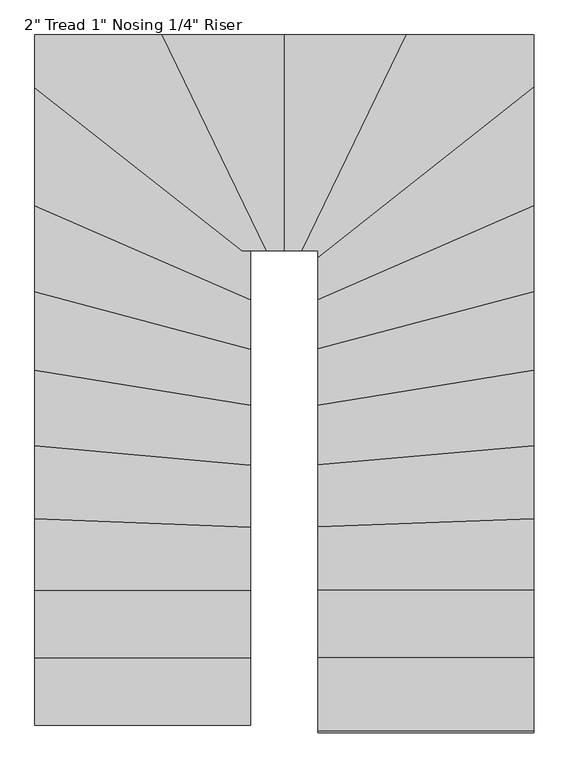
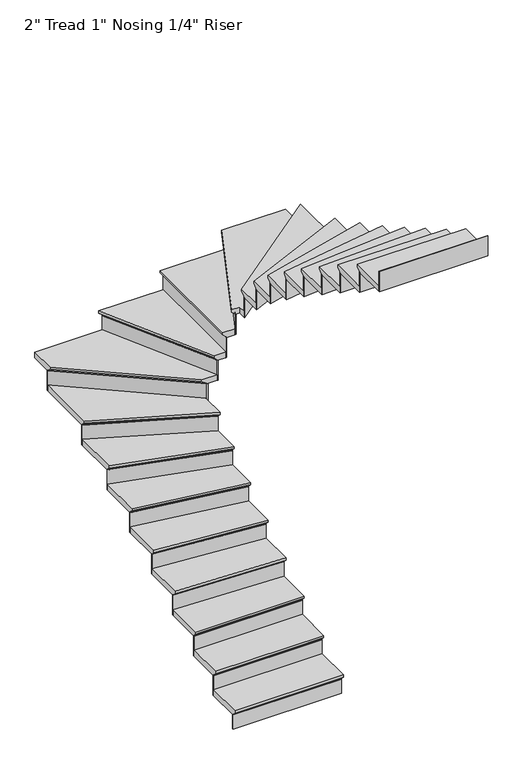
"""IFC4 building model written with IfcOpenShell, lengths in millimetres: stair flight geometry."""

from ifc_helpers import new_model, si_unit, origin, place, context, project, spatial, faceted_brep, source, transform, mapped, element, save


def stair_flight_836873dd(model_context):
    return source(origin(), model_context, "Body", "Brep", [
        faceted_brep([(-5047.1987704, -4554.2130548, 3812.7214286), (-5047.1987704, -4554.2130548, 3831.7714286), (-5940.8822214, -4554.2130548, 3831.7714286), (-5940.8822214, -4554.2130548, 3812.7214286), (-5047.1987704, -4528.8130548, 3787.3214286), (-5940.8822214, -4528.8130548, 3787.3214286), (-5047.1987704, -4249.4130548, 3831.7714286), (-5940.8822214, -4249.4130548, 3831.7714286), (-5940.8822214, -4528.8130548, 3780.9714286), (-5940.8822214, -4249.4130548, 3780.9714286), (-5047.1987704, -4249.4130548, 3780.9714286), (-5047.1987704, -4528.8130548, 3780.9714286)], [[[0, 1, 2, 3]], [[4, 0, 3, 5]], [[2, 1, 6, 7]], [[8, 9, 10, 11]], [[2, 7, 9, 8, 5, 3]], [[8, 11, 4, 5]], [[6, 1, 0, 4, 11, 10]], [[7, 6, 10, 9]]]),
        faceted_brep([(-5047.1987704, -4528.8130548, 3780.9714286), (-5047.1987704, -4528.8130548, 3657.6), (-5047.1987704, -4522.4630548, 3657.6), (-5047.1987704, -4522.4630548, 3780.9714286), (-5940.8822214, -4528.8130548, 3780.9714286), (-5940.8822214, -4522.4630548, 3780.9714286), (-5940.8822214, -4522.4630548, 3657.6), (-5940.8822214, -4528.8130548, 3657.6)], [[[0, 1, 2, 3]], [[4, 5, 6, 7]], [[1, 0, 4, 7]], [[2, 1, 7, 6]], [[3, 2, 6, 5]], [[0, 3, 5, 4]]]),
        faceted_brep([(-5047.1987704, -4249.4130548, 3955.1428571), (-5047.1987704, -4249.4130548, 3780.9714286), (-5047.1987704, -4243.0630548, 3780.9714286), (-5047.1987704, -4243.0630548, 3955.1428571), (-5940.8822214, -4249.4130548, 3955.1428571), (-5940.8822214, -4243.0630548, 3955.1428571), (-5940.8822214, -4243.0630548, 3780.9714286), (-5940.8822214, -4249.4130548, 3780.9714286)], [[[0, 1, 2, 3]], [[4, 5, 6, 7]], [[1, 0, 4, 7]], [[2, 1, 7, 6]], [[3, 2, 6, 5]], [[0, 3, 5, 4]]]),
        faceted_brep([(-5940.8822214, -4274.8130548, 4005.9428571), (-5047.1987704, -4274.8130548, 4005.9428571), (-5047.1987704, -3970.0130548, 4005.9428571), (-5940.8822214, -3970.0130548, 4005.9428571), (-5940.8822214, -4249.4130548, 3955.1428571), (-5940.8822214, -3970.0130548, 3955.1428571), (-5047.1987704, -3970.0130548, 3955.1428571), (-5047.1987704, -4249.4130548, 3955.1428571), (-5940.8822214, -4249.4130548, 3961.4928571), (-5940.8822214, -4274.8130548, 3986.8928571), (-5047.1987704, -4249.4130548, 3961.4928571), (-5047.1987704, -4274.8130548, 3986.8928571)], [[[0, 1, 2, 3]], [[4, 5, 6, 7]], [[0, 3, 5, 4, 8, 9]], [[4, 7, 10, 8]], [[2, 1, 11, 10, 7, 6]], [[3, 2, 6, 5]], [[11, 1, 0, 9]], [[10, 11, 9, 8]]]),
        faceted_brep([(-5047.1987704, -3970.0130548, 4129.3142857), (-5047.1987704, -3970.0130548, 3955.1428571), (-5047.1987704, -3963.6630548, 3955.1428571), (-5047.1987704, -3963.6630548, 4129.3142857), (-5940.8822214, -3970.0130548, 4129.3142857), (-5940.8822214, -3963.6630548, 4129.3142857), (-5940.8822214, -3963.6630548, 3955.1428571), (-5940.8822214, -3970.0130548, 3955.1428571)], [[[0, 1, 2, 3]], [[4, 5, 6, 7]], [[1, 0, 4, 7]], [[2, 1, 7, 6]], [[3, 2, 6, 5]], [[0, 3, 5, 4]]]),
        faceted_brep([(-5940.8822214, -3995.4130548, 4180.1142857), (-5047.1987704, -3995.4130548, 4180.1142857), (-5047.1987704, -3707.9036879, 4180.1142857), (-5940.8822214, -3673.2843203, 4180.1142857), (-5940.8822214, -3970.0130548, 4129.3142857), (-5940.8822214, -3673.2843203, 4129.3142857), (-5047.1987704, -3707.9036879, 4129.3142857), (-5047.1987704, -3970.0130548, 4129.3142857), (-5940.8822214, -3970.0130548, 4135.6642857), (-5940.8822214, -3995.4130548, 4161.0642857), (-5047.1987704, -3970.0130548, 4135.6642857), (-5047.1987704, -3995.4130548, 4161.0642857)], [[[0, 1, 2, 3]], [[4, 5, 6, 7]], [[0, 3, 5, 4, 8, 9]], [[4, 7, 10, 8]], [[2, 1, 11, 10, 7, 6]], [[3, 2, 6, 5]], [[11, 1, 0, 9]], [[10, 11, 9, 8]]]),
        faceted_brep([(-5047.1987704, -3707.9036879, 4303.4857143), (-5047.1987704, -3707.9036879, 4129.3142857), (-5047.1987704, -3701.5489252, 4129.3142857), (-5047.1987704, -3701.5489252, 4303.4857143), (-5940.8822214, -3673.2843203, 4303.4857143), (-5940.8822214, -3666.9295576, 4303.4857143), (-5940.8822214, -3666.9295576, 4129.3142857), (-5940.8822214, -3673.2843203, 4129.3142857)], [[[0, 1, 2, 3]], [[4, 5, 6, 7]], [[1, 0, 4, 7]], [[2, 1, 7, 6]], [[3, 2, 6, 5]], [[0, 3, 5, 4]]]),
        faceted_brep([(-5940.8822214, -3698.703371, 4354.2857143), (-5047.1987704, -3733.3227386, 4354.2857143), (-5047.1987704, -3451.3234819, 4354.2857143), (-5940.8822214, -3370.89733, 4354.2857143), (-5940.8822214, -3673.2843203, 4303.4857143), (-5940.8822214, -3370.89733, 4303.4857143), (-5047.1987704, -3451.3234819, 4303.4857143), (-5047.1987704, -3707.9036879, 4303.4857143), (-5940.8822214, -3673.2843203, 4309.8357143), (-5940.8822214, -3698.703371, 4335.2357143), (-5047.1987704, -3707.9036879, 4309.8357143), (-5047.1987704, -3733.3227386, 4335.2357143)], [[[0, 1, 2, 3]], [[4, 5, 6, 7]], [[0, 3, 5, 4, 8, 9]], [[4, 7, 10, 8]], [[2, 1, 11, 10, 7, 6]], [[3, 2, 6, 5]], [[11, 1, 0, 9]], [[10, 11, 9, 8]]]),
        faceted_brep([(-5047.1987704, -3451.3234819, 4477.6571429), (-5047.1987704, -3451.3234819, 4303.4857143), (-5047.1987704, -3444.9478197, 4303.4857143), (-5047.1987704, -3444.9478197, 4477.6571429), (-5940.8822214, -3370.89733, 4477.6571429), (-5940.8822214, -3364.5216678, 4477.6571429), (-5940.8822214, -3364.5216678, 4303.4857143), (-5940.8822214, -3370.89733, 4303.4857143)], [[[0, 1, 2, 3]], [[4, 5, 6, 7]], [[1, 0, 4, 7]], [[2, 1, 7, 6]], [[3, 2, 6, 5]], [[0, 3, 5, 4]]]),
        faceted_brep([(-5940.8822214, -3396.3999789, 4528.4571429), (-5047.1987704, -3476.8261308, 4528.4571429), (-5047.1987704, -3203.4301079, 4528.4571429), (-5940.8822214, -3059.5417727, 4528.4571429), (-5940.8822214, -3370.89733, 4477.6571429), (-5940.8822214, -3059.5417727, 4477.6571429), (-5047.1987704, -3203.4301079, 4477.6571429), (-5047.1987704, -3451.3234819, 4477.6571429), (-5940.8822214, -3370.89733, 4484.0071429), (-5940.8822214, -3396.3999789, 4509.4071429), (-5047.1987704, -3451.3234819, 4484.0071429), (-5047.1987704, -3476.8261308, 4509.4071429)], [[[0, 1, 2, 3]], [[4, 5, 6, 7]], [[0, 3, 5, 4, 8, 9]], [[4, 7, 10, 8]], [[2, 1, 11, 10, 7, 6]], [[3, 2, 6, 5]], [[11, 1, 0, 9]], [[10, 11, 9, 8]]]),
        faceted_brep([(-5047.1987704, -3203.4301079, 4651.8285714), (-5047.1987704, -3203.4301079, 4477.6571429), (-5047.1987704, -3196.9983292, 4477.6571429), (-5047.1987704, -3196.9983292, 4651.8285714), (-5940.8822214, -3059.5417727, 4651.8285714), (-5940.8822214, -3053.109994, 4651.8285714), (-5940.8822214, -3053.109994, 4477.6571429), (-5940.8822214, -3059.5417727, 4477.6571429)], [[[0, 1, 2, 3]], [[4, 5, 6, 7]], [[1, 0, 4, 7]], [[2, 1, 7, 6]], [[3, 2, 6, 5]], [[0, 3, 5, 4]]]),
        faceted_brep([(-5940.8822214, -3085.2688872, 4702.6285714), (-5047.1987704, -3229.1572224, 4702.6285714), (-5047.1987704, -2970.3553609, 4702.6285714), (-5940.8822214, -2732.7052783, 4702.6285714), (-5940.8822214, -3059.5417727, 4651.8285714), (-5940.8822214, -2732.7052783, 4651.8285714), (-5047.1987704, -2970.3553609, 4651.8285714), (-5047.1987704, -3203.4301079, 4651.8285714), (-5940.8822214, -3059.5417727, 4658.1785714), (-5940.8822214, -3085.2688872, 4683.5785714), (-5047.1987704, -3203.4301079, 4658.1785714), (-5047.1987704, -3229.1572224, 4683.5785714)], [[[0, 1, 2, 3]], [[4, 5, 6, 7]], [[0, 3, 5, 4, 8, 9]], [[4, 7, 10, 8]], [[2, 1, 11, 10, 7, 6]], [[3, 2, 6, 5]], [[11, 1, 0, 9]], [[10, 11, 9, 8]]]),
        faceted_brep([(-5047.1987704, -2970.3553609, 4826.0), (-5047.1987704, -2970.3553609, 4651.8285714), (-5047.1987704, -2963.7846771, 4651.8285714), (-5047.1987704, -2963.7846771, 4826.0), (-5940.8822214, -2732.7052783, 4826.0), (-5940.8822214, -2726.1345945, 4826.0), (-5940.8822214, -2726.1345945, 4651.8285714), (-5940.8822214, -2732.7052783, 4651.8285714)], [[[0, 1, 2, 3]], [[4, 5, 6, 7]], [[1, 0, 4, 7]], [[2, 1, 7, 6]], [[3, 2, 6, 5]], [[0, 3, 5, 4]]]),
        faceted_brep([(-5940.8822214, -2758.9880136, 4876.8), (-5047.1987704, -2996.6380961, 4876.8), (-5047.1987704, -2765.8050203, 4876.8), (-5940.8822214, -2375.5896532, 4876.8), (-5940.8822214, -2732.7052783, 4826.0), (-5940.8822214, -2375.5896532, 4826.0), (-5047.1987704, -2765.8050203, 4826.0), (-5047.1987704, -2970.3553609, 4826.0), (-5940.8822214, -2732.7052783, 4832.35), (-5940.8822214, -2758.9880136, 4857.75), (-5047.1987704, -2970.3553609, 4832.35), (-5047.1987704, -2996.6380961, 4857.75)], [[[0, 1, 2, 3]], [[4, 5, 6, 7]], [[0, 3, 5, 4, 8, 9]], [[4, 7, 10, 8]], [[2, 1, 11, 10, 7, 6]], [[3, 2, 6, 5]], [[11, 1, 0, 9]], [[10, 11, 9, 8]]]),
        faceted_brep([(-5047.1987704, -2765.8050203, 5000.1714286), (-5047.1987704, -2765.8050203, 4826.0), (-5047.1987704, -2758.8760908, 4826.0), (-5047.1987704, -2758.8760908, 5000.1714286), (-5940.8822214, -2375.5896532, 5000.1714286), (-5940.8822214, -2368.6607237, 5000.1714286), (-5940.8822214, -2368.6607237, 4826.0), (-5940.8822214, -2375.5896532, 4826.0)], [[[0, 1, 2, 3]], [[4, 5, 6, 7]], [[1, 0, 4, 7]], [[2, 1, 7, 6]], [[3, 2, 6, 5]], [[0, 3, 5, 4]]]),
        faceted_brep([(-5940.8822214, -2403.3053713, 5050.9714286), (-5047.1987704, -2793.5207384, 5050.9714286), (-5047.1987704, -2590.8424524, 5050.9714286), (-5040.8038639, -2590.8424524, 5050.9714286), (-5940.8822214, -1882.1944717, 5050.9714286), (-5940.8822214, -2375.5896532, 5000.1714286), (-5940.8822214, -1882.1944717, 5000.1714286), (-5040.8038639, -2590.8424524, 5000.1714286), (-5047.1987704, -2590.8424524, 5000.1714286), (-5047.1987704, -2765.8050203, 5000.1714286), (-5940.8822214, -2375.5896532, 5006.5214286), (-5940.8822214, -2403.3053713, 5031.9214286), (-5047.1987704, -2765.8050203, 5006.5214286), (-5047.1987704, -2793.5207384, 5031.9214286)], [[[0, 1, 2, 3, 4]], [[5, 6, 7, 8, 9]], [[0, 4, 6, 5, 10, 11]], [[5, 9, 12, 10]], [[2, 1, 13, 12, 9, 8]], [[4, 3, 7, 6]], [[13, 1, 0, 11]], [[12, 13, 11, 10]], [[3, 2, 8, 7]]]),
        faceted_brep([(-5040.8038639, -2590.8424524, 5174.3428571), (-5040.8038639, -2590.8424524, 5000.1714286), (-5030.5387554, -2590.8424524, 5000.1714286), (-5030.5387554, -2590.8424524, 5174.3428571), (-5940.8822214, -1882.1944717, 5174.3428571), (-5940.8822214, -1874.1125661, 5174.3428571), (-5940.8822214, -1874.1125661, 5000.1714286), (-5940.8822214, -1882.1944717, 5000.1714286)], [[[0, 1, 2, 3]], [[4, 5, 6, 7]], [[1, 0, 4, 7]], [[2, 1, 7, 6]], [[3, 2, 6, 5]], [[0, 3, 5, 4]]]),
        faceted_brep([(-5384.6489457, -1697.1590014, 5225.1428571), (-5940.8822214, -1697.1590014, 5225.1428571), (-5940.8822214, -1914.5220945, 5225.1428571), (-5081.8642978, -2590.8424524, 5225.1428571), (-4952.3566185, -2590.8424524, 5225.1428571), (-5940.8822214, -1697.1590014, 5174.3428571), (-5384.6489457, -1697.1590014, 5174.3428571), (-4952.3566185, -2590.8424524, 5174.3428571), (-5040.8038639, -2590.8424524, 5174.3428571), (-5940.8822214, -1882.1944717, 5174.3428571), (-5940.8822214, -1882.1944717, 5180.6928571), (-5940.8822214, -1914.5220945, 5206.0928571), (-5040.8038639, -2590.8424524, 5180.6928571), (-5081.8642978, -2590.8424524, 5206.0928571)], [[[0, 1, 2, 3, 4]], [[5, 6, 7, 8, 9]], [[1, 0, 6, 5]], [[2, 1, 5, 9, 10, 11]], [[9, 8, 12, 10]], [[4, 3, 13, 12, 8, 7]], [[0, 4, 7, 6]], [[13, 3, 2, 11]], [[12, 13, 11, 10]]]),
        faceted_brep([(-4952.3566185, -2590.8424524, 5348.5142857), (-4952.3566185, -2590.8424524, 5174.3428571), (-4945.3027294, -2590.8424524, 5174.3428571), (-4945.3027294, -2590.8424524, 5348.5142857), (-5384.6489457, -1697.1590014, 5348.5142857), (-5377.5950566, -1697.1590014, 5348.5142857), (-5377.5950566, -1697.1590014, 5174.3428571), (-5384.6489457, -1697.1590014, 5174.3428571)], [[[0, 1, 2, 3]], [[4, 5, 6, 7]], [[1, 0, 4, 7]], [[2, 1, 7, 6]], [[3, 2, 6, 5]], [[0, 3, 5, 4]]]),
        faceted_brep([(-5412.8645022, -1697.1590014, 5399.3142857), (-4980.5721749, -2590.8424524, 5399.3142857), (-4882.0987704, -2590.8424524, 5399.3142857), (-4882.0987706, -1697.1590014, 5399.3142857), (-5384.6489457, -1697.1590014, 5348.5142857), (-4882.0987706, -1697.1590014, 5348.5142857), (-4882.0987704, -2590.8424524, 5348.5142857), (-4952.3566185, -2590.8424524, 5348.5142857), (-5384.6489457, -1697.1590014, 5354.8642857), (-5412.8645022, -1697.1590014, 5380.2642857), (-4952.3566185, -2590.8424524, 5354.8642857), (-4980.5721749, -2590.8424524, 5380.2642857)], [[[0, 1, 2, 3]], [[4, 5, 6, 7]], [[0, 3, 5, 4, 8, 9]], [[4, 7, 10, 8]], [[3, 2, 6, 5]], [[11, 1, 0, 9]], [[10, 11, 9, 8]], [[2, 1, 11, 10, 7, 6]]]),
        faceted_brep([(-4882.0987704, -2590.8424524, 5522.6857143), (-4882.0987704, -2590.8424524, 5348.5142857), (-4875.7487704, -2590.8424524, 5348.5142857), (-4875.7487704, -2590.8424524, 5522.6857143), (-4882.0987706, -1697.1590014, 5522.6857143), (-4875.7487706, -1697.1590014, 5522.6857143), (-4875.7487706, -1697.1590014, 5348.5142857), (-4882.0987706, -1697.1590014, 5348.5142857)], [[[0, 1, 2, 3]], [[4, 5, 6, 7]], [[1, 0, 4, 7]], [[2, 1, 7, 6]], [[3, 2, 6, 5]], [[0, 3, 5, 4]]]),
        faceted_brep([(-4907.4987706, -1697.1590014, 5573.4857143), (-4907.4987704, -2590.8424524, 5573.4857143), (-4806.2098095, -2590.8424524, 5573.4857143), (-4373.9174828, -1697.1590014, 5573.4857143), (-4882.0987706, -1697.1590014, 5522.6857143), (-4373.9174828, -1697.1590014, 5522.6857143), (-4806.2098095, -2590.8424524, 5522.6857143), (-4882.0987704, -2590.8424524, 5522.6857143), (-4882.0987706, -1697.1590014, 5529.0357143), (-4907.4987706, -1697.1590014, 5554.4357143), (-4882.0987704, -2590.8424524, 5529.0357143), (-4907.4987704, -2590.8424524, 5554.4357143)], [[[0, 1, 2, 3]], [[4, 5, 6, 7]], [[0, 3, 5, 4, 8, 9]], [[4, 7, 10, 8]], [[2, 1, 11, 10, 7, 6]], [[3, 2, 6, 5]], [[11, 1, 0, 9]], [[10, 11, 9, 8]]]),
        faceted_brep([(-4806.2098095, -2590.8424524, 5696.8571429), (-4806.2098095, -2590.8424524, 5522.6857143), (-4799.1559204, -2590.8424524, 5522.6857143), (-4799.1559204, -2590.8424524, 5696.8571429), (-4373.9174828, -1697.1590014, 5696.8571429), (-4366.8635937, -1697.1590014, 5696.8571429), (-4366.8635937, -1697.1590014, 5522.6857143), (-4373.9174828, -1697.1590014, 5522.6857143)], [[[0, 1, 2, 3]], [[4, 5, 6, 7]], [[1, 0, 4, 7]], [[2, 1, 7, 6]], [[3, 2, 6, 5]], [[0, 3, 5, 4]]]),
        faceted_brep([(-3874.1153195, -1946.8497166, 5747.6571429), (-3874.1153195, -1697.1590014, 5747.6571429), (-4402.1330392, -1697.1590014, 5747.6571429), (-4834.4253659, -2590.8424524, 5747.6571429), (-4767.7987704, -2590.8424524, 5747.6571429), (-4767.7987704, -2650.4628721, 5747.6571429), (-3874.1153195, -1697.1590014, 5696.8571429), (-3874.1153195, -1946.8497166, 5696.8571429), (-4767.7987704, -2650.4628721, 5696.8571429), (-4767.7987704, -2590.8424524, 5696.8571429), (-4806.2098095, -2590.8424524, 5696.8571429), (-4373.9174828, -1697.1590014, 5696.8571429), (-4806.2098095, -2590.8424524, 5703.2071429), (-4373.9174828, -1697.1590014, 5703.2071429), (-4834.4253659, -2590.8424524, 5728.6071429), (-4402.1330392, -1697.1590014, 5728.6071429)], [[[0, 1, 2, 3, 4, 5]], [[6, 7, 8, 9, 10, 11]], [[1, 0, 7, 6]], [[11, 10, 12, 13]], [[4, 3, 14, 12, 10, 9]], [[5, 4, 9, 8]], [[0, 5, 8, 7]], [[14, 3, 2, 15]], [[12, 14, 15, 13]], [[2, 1, 6, 11, 13, 15]]]),
        faceted_brep([(-4767.7987704, -2650.4628721, 5871.0285714), (-4767.7987704, -2650.4628721, 5696.8571429), (-4767.7987704, -2658.5447778, 5696.8571429), (-4767.7987704, -2658.5447778, 5871.0285714), (-3874.1153195, -1946.8497166, 5871.0285714), (-3874.1153195, -1954.9316222, 5871.0285714), (-3874.1153195, -1954.9316222, 5696.8571429), (-3874.1153195, -1946.8497166, 5696.8571429)], [[[0, 1, 2, 3]], [[4, 5, 6, 7]], [[1, 0, 4, 7]], [[2, 1, 7, 6]], [[3, 2, 6, 5]], [[0, 3, 5, 4]]]),
        faceted_brep([(-3874.1153195, -1914.5220938, 5921.8285714), (-4767.7987704, -2618.1352494, 5921.8285714), (-4767.7987704, -2821.2364563, 5921.8285714), (-3874.1153195, -2431.0210889, 5921.8285714), (-3874.1153195, -1946.8497166, 5871.0285714), (-3874.1153195, -2431.0210889, 5871.0285714), (-4767.7987704, -2821.2364563, 5871.0285714), (-4767.7987704, -2650.4628721, 5871.0285714), (-3874.1153195, -1946.8497166, 5877.3785714), (-3874.1153195, -1914.5220938, 5902.7785714), (-4767.7987704, -2650.4628721, 5877.3785714), (-4767.7987704, -2618.1352494, 5902.7785714)], [[[0, 1, 2, 3]], [[4, 5, 6, 7]], [[0, 3, 5, 4, 8, 9]], [[4, 7, 10, 8]], [[2, 1, 11, 10, 7, 6]], [[3, 2, 6, 5]], [[11, 1, 0, 9]], [[10, 11, 9, 8]]]),
        faceted_brep([(-4767.7987704, -2821.2364563, 6045.2), (-4767.7987704, -2821.2364563, 5871.0285714), (-4767.7987704, -2828.1653858, 5871.0285714), (-4767.7987704, -2828.1653858, 6045.2), (-3874.1153195, -2431.0210889, 6045.2), (-3874.1153195, -2437.9500185, 6045.2), (-3874.1153195, -2437.9500185, 5871.0285714), (-3874.1153195, -2431.0210889, 5871.0285714)], [[[0, 1, 2, 3]], [[4, 5, 6, 7]], [[1, 0, 4, 7]], [[2, 1, 7, 6]], [[3, 2, 6, 5]], [[0, 3, 5, 4]]]),
        faceted_brep([(-3874.1153195, -2403.3053709, 6096.0), (-4767.7987704, -2793.5207382, 6096.0), (-4767.7987704, -3022.9208311, 6096.0), (-3874.1153195, -2785.2707484, 6096.0), (-3874.1153195, -2431.0210889, 6045.2), (-3874.1153195, -2785.2707484, 6045.2), (-4767.7987704, -3022.9208311, 6045.2), (-4767.7987704, -2821.2364563, 6045.2), (-3874.1153195, -2431.0210889, 6051.55), (-3874.1153195, -2403.3053709, 6076.95), (-4767.7987704, -2821.2364563, 6051.55), (-4767.7987704, -2793.5207382, 6076.95)], [[[0, 1, 2, 3]], [[4, 5, 6, 7]], [[0, 3, 5, 4, 8, 9]], [[4, 7, 10, 8]], [[2, 1, 11, 10, 7, 6]], [[3, 2, 6, 5]], [[11, 1, 0, 9]], [[10, 11, 9, 8]]]),
        faceted_brep([(-4767.7987704, -3022.9208311, 6219.3714286), (-4767.7987704, -3022.9208311, 6045.2), (-4767.7987704, -3029.4915149, 6045.2), (-4767.7987704, -3029.4915149, 6219.3714286), (-3874.1153195, -2785.2707484, 6219.3714286), (-3874.1153195, -2791.8414322, 6219.3714286), (-3874.1153195, -2791.8414322, 6045.2), (-3874.1153195, -2785.2707484, 6045.2)], [[[0, 1, 2, 3]], [[4, 5, 6, 7]], [[1, 0, 4, 7]], [[2, 1, 7, 6]], [[3, 2, 6, 5]], [[0, 3, 5, 4]]]),
        faceted_brep([(-3874.1153195, -2758.9880132, 6270.1714286), (-4767.7987704, -2996.6380959, 6270.1714286), (-4767.7987704, -3254.8843368, 6270.1714286), (-3874.1153195, -3110.9960015, 6270.1714286), (-3874.1153195, -2785.2707484, 6219.3714286), (-3874.1153195, -3110.9960015, 6219.3714286), (-4767.7987704, -3254.8843368, 6219.3714286), (-4767.7987704, -3022.9208311, 6219.3714286), (-3874.1153195, -2785.2707484, 6225.7214286), (-3874.1153195, -2758.9880132, 6251.1214286), (-4767.7987704, -3022.9208311, 6225.7214286), (-4767.7987704, -2996.6380959, 6251.1214286)], [[[0, 1, 2, 3]], [[4, 5, 6, 7]], [[0, 3, 5, 4, 8, 9]], [[4, 7, 10, 8]], [[2, 1, 11, 10, 7, 6]], [[3, 2, 6, 5]], [[11, 1, 0, 9]], [[10, 11, 9, 8]]]),
        faceted_brep([(-4767.7987704, -3254.8843368, 6393.5428571), (-4767.7987704, -3254.8843368, 6219.3714286), (-4767.7987704, -3261.3161154, 6219.3714286), (-4767.7987704, -3261.3161154, 6393.5428571), (-3874.1153195, -3110.9960015, 6393.5428571), (-3874.1153195, -3117.4277801, 6393.5428571), (-3874.1153195, -3117.4277801, 6219.3714286), (-3874.1153195, -3110.9960015, 6219.3714286)], [[[0, 1, 2, 3]], [[4, 5, 6, 7]], [[1, 0, 4, 7]], [[2, 1, 7, 6]], [[3, 2, 6, 5]], [[0, 3, 5, 4]]]),
        faceted_brep([(-3874.1153195, -3085.2688869, 6444.3428571), (-4767.7987704, -3229.1572222, 6444.3428571), (-4767.7987704, -3502.3287795, 6444.3428571), (-3874.1153195, -3421.9026274, 6444.3428571), (-3874.1153195, -3110.9960015, 6393.5428571), (-3874.1153195, -3421.9026274, 6393.5428571), (-4767.7987704, -3502.3287795, 6393.5428571), (-4767.7987704, -3254.8843368, 6393.5428571), (-3874.1153195, -3110.9960015, 6399.8928571), (-3874.1153195, -3085.2688869, 6425.2928571), (-4767.7987704, -3254.8843368, 6399.8928571), (-4767.7987704, -3229.1572222, 6425.2928571)], [[[0, 1, 2, 3]], [[4, 5, 6, 7]], [[0, 3, 5, 4, 8, 9]], [[4, 7, 10, 8]], [[2, 1, 11, 10, 7, 6]], [[3, 2, 6, 5]], [[11, 1, 0, 9]], [[10, 11, 9, 8]]]),
        faceted_brep([(-4767.7987704, -3502.3287795, 6567.7142857), (-4767.7987704, -3502.3287795, 6393.5428571), (-4767.7987704, -3508.7044417, 6393.5428571), (-4767.7987704, -3508.7044417, 6567.7142857), (-3874.1153195, -3421.9026274, 6567.7142857), (-3874.1153195, -3428.2782897, 6567.7142857), (-3874.1153195, -3428.2782897, 6393.5428571), (-3874.1153195, -3421.9026274, 6393.5428571)], [[[0, 1, 2, 3]], [[4, 5, 6, 7]], [[1, 0, 4, 7]], [[2, 1, 7, 6]], [[3, 2, 6, 5]], [[0, 3, 5, 4]]]),
        faceted_brep([(-3874.1153195, -3396.3999786, 6618.5142857), (-4767.7987704, -3476.8261306, 6618.5142857), (-4767.7987704, -3758.7417891, 6618.5142857), (-3874.1153195, -3724.1224215, 6618.5142857), (-3874.1153195, -3421.9026274, 6567.7142857), (-3874.1153195, -3724.1224215, 6567.7142857), (-4767.7987704, -3758.7417891, 6567.7142857), (-4767.7987704, -3502.3287795, 6567.7142857), (-3874.1153195, -3421.9026274, 6574.0642857), (-3874.1153195, -3396.3999786, 6599.4642857), (-4767.7987704, -3502.3287795, 6574.0642857), (-4767.7987704, -3476.8261306, 6599.4642857)], [[[0, 1, 2, 3]], [[4, 5, 6, 7]], [[0, 3, 5, 4, 8, 9]], [[4, 7, 10, 8]], [[2, 1, 11, 10, 7, 6]], [[3, 2, 6, 5]], [[11, 1, 0, 9]], [[10, 11, 9, 8]]]),
        faceted_brep([(-4767.7987704, -3758.7417891, 6741.8857143), (-4767.7987704, -3758.7417891, 6567.7142857), (-4767.7987704, -3765.0965518, 6567.7142857), (-4767.7987704, -3765.0965518, 6741.8857143), (-3874.1153195, -3724.1224215, 6741.8857143), (-3874.1153195, -3730.4771842, 6741.8857143), (-3874.1153195, -3730.4771842, 6567.7142857), (-3874.1153195, -3724.1224215, 6567.7142857)], [[[0, 1, 2, 3]], [[4, 5, 6, 7]], [[1, 0, 4, 7]], [[2, 1, 7, 6]], [[3, 2, 6, 5]], [[0, 3, 5, 4]]]),
        faceted_brep([(-3874.1153195, -3698.7033708, 6792.6857143), (-4767.7987704, -3733.3227384, 6792.6857143), (-4767.7987704, -4020.8130546, 6792.6857143), (-3874.1153195, -4020.8130546, 6792.6857143), (-3874.1153195, -3724.1224215, 6741.8857143), (-3874.1153195, -4020.8130546, 6741.8857143), (-4767.7987704, -4020.8130546, 6741.8857143), (-4767.7987704, -3758.7417891, 6741.8857143), (-3874.1153195, -3724.1224215, 6748.2357143), (-3874.1153195, -3698.7033708, 6773.6357143), (-4767.7987704, -3758.7417891, 6748.2357143), (-4767.7987704, -3733.3227384, 6773.6357143)], [[[0, 1, 2, 3]], [[4, 5, 6, 7]], [[0, 3, 5, 4, 8, 9]], [[4, 7, 10, 8]], [[2, 1, 11, 10, 7, 6]], [[3, 2, 6, 5]], [[11, 1, 0, 9]], [[10, 11, 9, 8]]]),
        faceted_brep([(-4767.7987704, -4020.8130546, 6916.0571429), (-4767.7987704, -4020.8130546, 6741.8857143), (-4767.7987704, -4027.1630546, 6741.8857143), (-4767.7987704, -4027.1630546, 6916.0571429), (-3874.1153195, -4020.8130546, 6916.0571429), (-3874.1153195, -4027.1630546, 6916.0571429), (-3874.1153195, -4027.1630546, 6741.8857143), (-3874.1153195, -4020.8130546, 6741.8857143)], [[[0, 1, 2, 3]], [[4, 5, 6, 7]], [[1, 0, 4, 7]], [[2, 1, 7, 6]], [[3, 2, 6, 5]], [[0, 3, 5, 4]]]),
        faceted_brep([(-3874.1153195, -3995.4130546, 6966.8571429), (-4767.7987704, -3995.4130546, 6966.8571429), (-4767.7987704, -4300.2130546, 6966.8571429), (-3874.1153195, -4300.2130546, 6966.8571429), (-3874.1153195, -4020.8130546, 6916.0571429), (-3874.1153195, -4300.2130546, 6916.0571429), (-4767.7987704, -4300.2130546, 6916.0571429), (-4767.7987704, -4020.8130546, 6916.0571429), (-3874.1153195, -4020.8130546, 6922.4071429), (-3874.1153195, -3995.4130546, 6947.8071429), (-4767.7987704, -4020.8130546, 6922.4071429), (-4767.7987704, -3995.4130546, 6947.8071429)], [[[0, 1, 2, 3]], [[4, 5, 6, 7]], [[0, 3, 5, 4, 8, 9]], [[4, 7, 10, 8]], [[2, 1, 11, 10, 7, 6]], [[3, 2, 6, 5]], [[11, 1, 0, 9]], [[10, 11, 9, 8]]]),
        faceted_brep([(-4767.7987704, -4300.2130546, 7090.2285714), (-4767.7987704, -4300.2130546, 6916.0571429), (-4767.7987704, -4306.5630546, 6916.0571429), (-4767.7987704, -4306.5630546, 7090.2285714), (-3874.1153195, -4300.2130546, 7090.2285714), (-3874.1153195, -4306.5630546, 7090.2285714), (-3874.1153195, -4306.5630546, 6916.0571429), (-3874.1153195, -4300.2130546, 6916.0571429)], [[[0, 1, 2, 3]], [[4, 5, 6, 7]], [[1, 0, 4, 7]], [[2, 1, 7, 6]], [[3, 2, 6, 5]], [[0, 3, 5, 4]]]),
        faceted_brep([(-4767.7987704, -4579.6130546, 7264.4), (-4767.7987704, -4579.6130546, 7090.2285714), (-4767.7987704, -4585.9630546, 7090.2285714), (-4767.7987704, -4585.9630546, 7264.4), (-3874.1153195, -4579.6130546, 7264.4), (-3874.1153195, -4585.9630546, 7264.4), (-3874.1153195, -4585.9630546, 7090.2285714), (-3874.1153195, -4579.6130546, 7090.2285714)], [[[0, 1, 2, 3]], [[4, 5, 6, 7]], [[1, 0, 4, 7]], [[2, 1, 7, 6]], [[3, 2, 6, 5]], [[0, 3, 5, 4]]]),
        faceted_brep([(-3874.1153195, -4274.8130546, 7141.0285714), (-4767.7987704, -4274.8130546, 7141.0285714), (-4767.7987704, -4579.6130546, 7141.0285714), (-3874.1153195, -4579.6130546, 7141.0285714), (-3874.1153195, -4300.2130546, 7090.2285714), (-3874.1153195, -4579.6130546, 7090.2285714), (-4767.7987704, -4579.6130546, 7090.2285714), (-4767.7987704, -4300.2130546, 7090.2285714), (-3874.1153195, -4300.2130546, 7096.5785714), (-3874.1153195, -4274.8130546, 7121.9785714), (-4767.7987704, -4300.2130546, 7096.5785714), (-4767.7987704, -4274.8130546, 7121.9785714)], [[[0, 1, 2, 3]], [[4, 5, 6, 7]], [[0, 3, 5, 4, 8, 9]], [[4, 7, 10, 8]], [[2, 1, 11, 10, 7, 6]], [[3, 2, 6, 5]], [[11, 1, 0, 9]], [[10, 11, 9, 8]]]),
    ])


if __name__ == "__main__":
    model = new_model("IFC4")
    model_context = context("Model", 3, world=origin())
    ifc_project = project(units=[si_unit("LENGTHUNIT", "METRE", prefix="MILLI")], contexts=[model_context])
    site = spatial("IfcSite", under=ifc_project)
    building = spatial("IfcBuilding", under=site)
    placement = place(None, origin())
    stair_flight_shape = stair_flight_836873dd(model_context)
    element("IfcStairFlight", 1, ObjectType="2\" Tread 1\" Nosing 1/4\" Riser", at=placement, inside=building, context=model_context, shape_type="MappedRepresentation", body=[
        mapped(stair_flight_shape, transform((0.0, 0.0, 0.0), x_axis=(1.0, 0.0, 0.0), y_axis=(0.0, 1.0, 0.0), z_axis=(0.0, 0.0, 1.0))),
    ])
    save(model, "model.ifc")

# Revit data of these elements
# Element 1 (IfcStairFlight, "2\" Tread 1\" Nosing 1/4\" Riser")
#   Materials on its faces: "Tile, Porcelain, 4in"
# Materials
#   "Tile, Porcelain, 4in": class "Generic", colour RGB 89 87 158, transparency 0, Description = "Porcelain tile, 4\", white", Cost = 0
